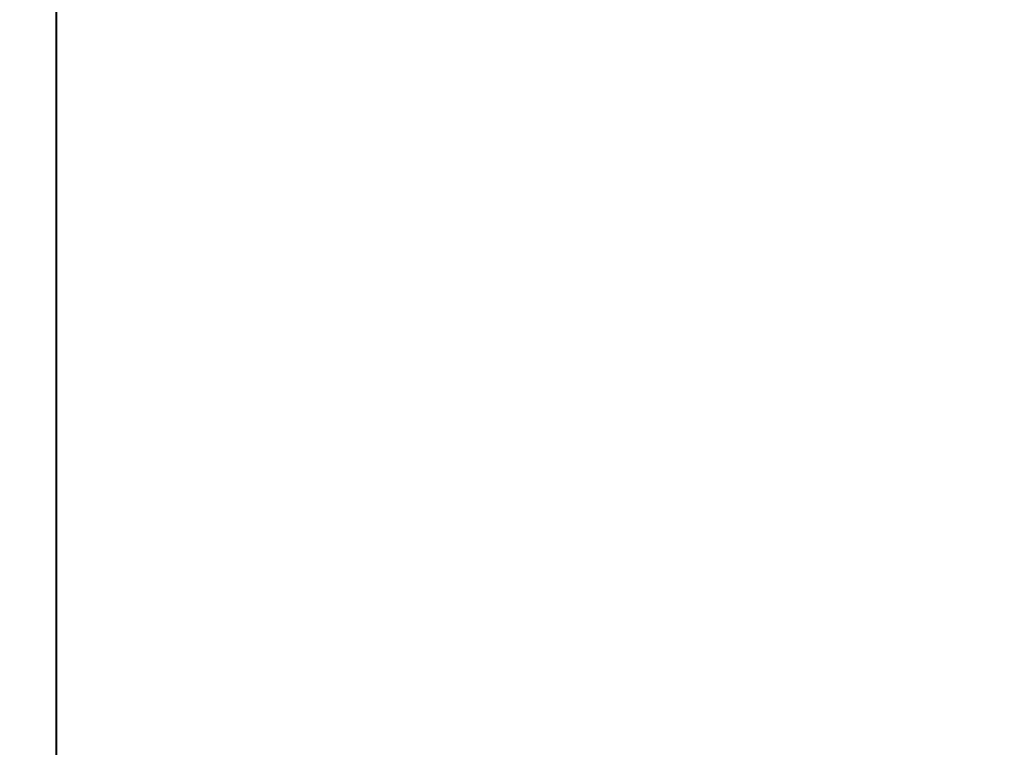
# Model space of a CAD drawing. Units: inches. Extents: x 459864 to 460310, y 324185 to 324787.
# Tile 93 of 112: x 460247.1043 to 460247.3904, y 324283.6409 to 324283.8523. Entities that reach past the tile are written whole.
import ezdxf

# ---------------------------------------------------------------- set-up
doc = ezdxf.new("R2010")
doc.units = ezdxf.units.IN
doc.layers.add('A-ANNO-DIMS', color=2, linetype='Continuous', lineweight=18)
doc.layers.add('A-WALL', color=7, linetype='Continuous', lineweight=40)
doc.styles.get("Standard").update_dxf_attribs({"font": 'arial.ttf'})
doc.dimstyles.new('ISO-25', dxfattribs={"dimtxt": 6, "dimasz": 2.5, "dimexe": 1.25, "dimexo": 0.625, "dimtad": 1, "dimdec": 1, "dimlunit": 3, "dimtxsty": 'Standard', "dimcen": 2.5, "dimadec": 0, "dimazin": 0, "dimtfac": 1, "dimtdec": 1, "dimtmove": 0, "dimatfit": 3, "dimfxl": 1, "dimarcsym": 0})

# ---------------------------------------------------------------- blocks, each defined once
blk = doc.blocks.new('*D21')
at = {"layer": 'A-ANNO-DIMS', "color": 0, "lineweight": -2, "transparency": 16777216}
for p, q in [((460247.73993, 324715.48323), (460309.58037, 324715.48323)), ((460308.33037, 324712.98323), (460308.33037, 324285.98323)), ((460247.73993, 324283.48323), (460309.58037, 324283.48323))]:
    blk.add_line(p, q, dxfattribs=at)
at = {"layer": 'A-ANNO-DIMS', "color": 0, "transparency": 16777216}
for points in [[(460307.9137, 324712.98323), (460308.74704, 324712.98323), (460308.33037, 324715.48323)], [(460307.9137, 324285.98323), (460308.74704, 324285.98323), (460308.33037, 324283.48323)]]:
    blk.add_solid(points, dxfattribs=at)
at = {"layer": 'Defpoints', "color": 0, "transparency": 16777216}
for p in [(460247.11493, 324715.48323), (460247.11493, 324283.48323), (460308.33037, 324283.48323)]:
    blk.add_point(p, dxfattribs=at)
at = {"layer": 'A-ANNO-DIMS', "color": 0, "transparency": 16777216, "insert": (460304.63988, 324499.48323), "char_height": 6, "attachment_point": 5, "rotation": 90}
blk.add_mtext("36'", dxfattribs=at)
blk = doc.blocks.new('*D62')
at = {"layer": 'A-ANNO-DIMS', "color": 0, "lineweight": -2, "transparency": 16777216}
for p, q in [((460247.73993, 324332.73872), (460278.76493, 324332.73872)), ((460277.51493, 324330.23872), (460277.51493, 324285.98323)), ((460247.73993, 324283.48323), (460278.76493, 324283.48323))]:
    blk.add_line(p, q, dxfattribs=at)
at = {"layer": 'A-ANNO-DIMS', "color": 0, "transparency": 16777216}
for points in [[(460277.09826, 324330.23872), (460277.93159, 324330.23872), (460277.51493, 324332.73872)], [(460277.09826, 324285.98323), (460277.93159, 324285.98323), (460277.51493, 324283.48323)]]:
    blk.add_solid(points, dxfattribs=at)
at = {"layer": 'Defpoints', "color": 0, "transparency": 16777216}
for p in [(460247.11493, 324332.73872), (460247.11493, 324283.48323), (460277.51493, 324283.48323)]:
    blk.add_point(p, dxfattribs=at)
at = {"layer": 'A-ANNO-DIMS', "color": 0, "transparency": 16777216, "insert": (460273.78761, 324308.11098), "char_height": 6, "attachment_point": 5, "rotation": 90}
blk.add_mtext('4\'-1 1/2"', dxfattribs=at)
blk = doc.blocks.new('*D67')
at = {"layer": 'A-ANNO-DIMS', "color": 0, "lineweight": -2, "transparency": 16777216}
for p, q in [((460208.11493, 324284.10823), (460208.11493, 324315.13323)), ((460247.11493, 324284.10823), (460247.11493, 324315.13323)), ((460210.61493, 324313.88323), (460244.61493, 324313.88323))]:
    blk.add_line(p, q, dxfattribs=at)
at = {"layer": 'A-ANNO-DIMS', "color": 0, "transparency": 16777216}
for points in [[(460210.61493, 324314.2999), (460210.61493, 324313.46657), (460208.11493, 324313.88323)], [(460244.61493, 324314.2999), (460244.61493, 324313.46657), (460247.11493, 324313.88323)]]:
    blk.add_solid(points, dxfattribs=at)
at = {"layer": 'Defpoints', "color": 0, "transparency": 16777216}
for p in [(460247.11493, 324313.88323), (460208.11493, 324283.48323), (460247.11493, 324283.48323)]:
    blk.add_point(p, dxfattribs=at)
at = {"layer": 'A-ANNO-DIMS', "color": 0, "transparency": 16777216, "insert": (460227.61493, 324317.57372), "char_height": 6, "attachment_point": 5}
blk.add_mtext('3\'-3"', dxfattribs=at)

msp = doc.modelspace()

# ---------------------------------------------------------------- linework, layer by layer
at = {"layer": 'A-WALL'}
msp.add_line((460247.11493, 324470.98323), (460247.11493, 324283.48323), dxfattribs=at)

# ---------------------------------------------------------------- dimensions: what is measured, and where the dimension line sits
at = {"layer": 'A-ANNO-DIMS'}
for base, p1, angle, override, picture, middle in [((460308.33037, 324283.48323), (460247.11493, 324715.48323), 90, {"dimclrd": 0, "dimclre": 0, "dimclrt": 0}, '*D21', (460304.63988, 324499.48323)), ((460277.51493, 324283.48323), (460247.11493, 324332.73872), 270, {"dimdec": 1, "dimlfac": 1, "dimrnd": 0, "dimzin": 1, "dimdsep": 46, "dimlunit": 4, "dimfrac": 2}, '*D62', (460273.78761, 324308.11098))]:
    dim = msp.add_linear_dim(base=base, p1=p1, p2=(460247.11493, 324283.48323), angle=angle, dimstyle='ISO-25', override=override, dxfattribs=at)
    dim.commit()
    dim.dimension.update_dxf_attribs({"geometry": picture, "text_midpoint": middle})
dim = msp.add_linear_dim(base=(460247.11493, 324313.88323), p1=(460208.11493, 324283.48323), p2=(460247.11493, 324283.48323), dimstyle='ISO-25', override={"dimdec": 1, "dimlfac": 1, "dimrnd": 0, "dimzin": 1, "dimdsep": 46, "dimlunit": 4, "dimfrac": 2}, dxfattribs=at)
dim.commit()
dim.dimension.update_dxf_attribs({"geometry": '*D67', "text_midpoint": (460227.61493, 324317.57372)})

doc.saveas('drawing.dxf')
